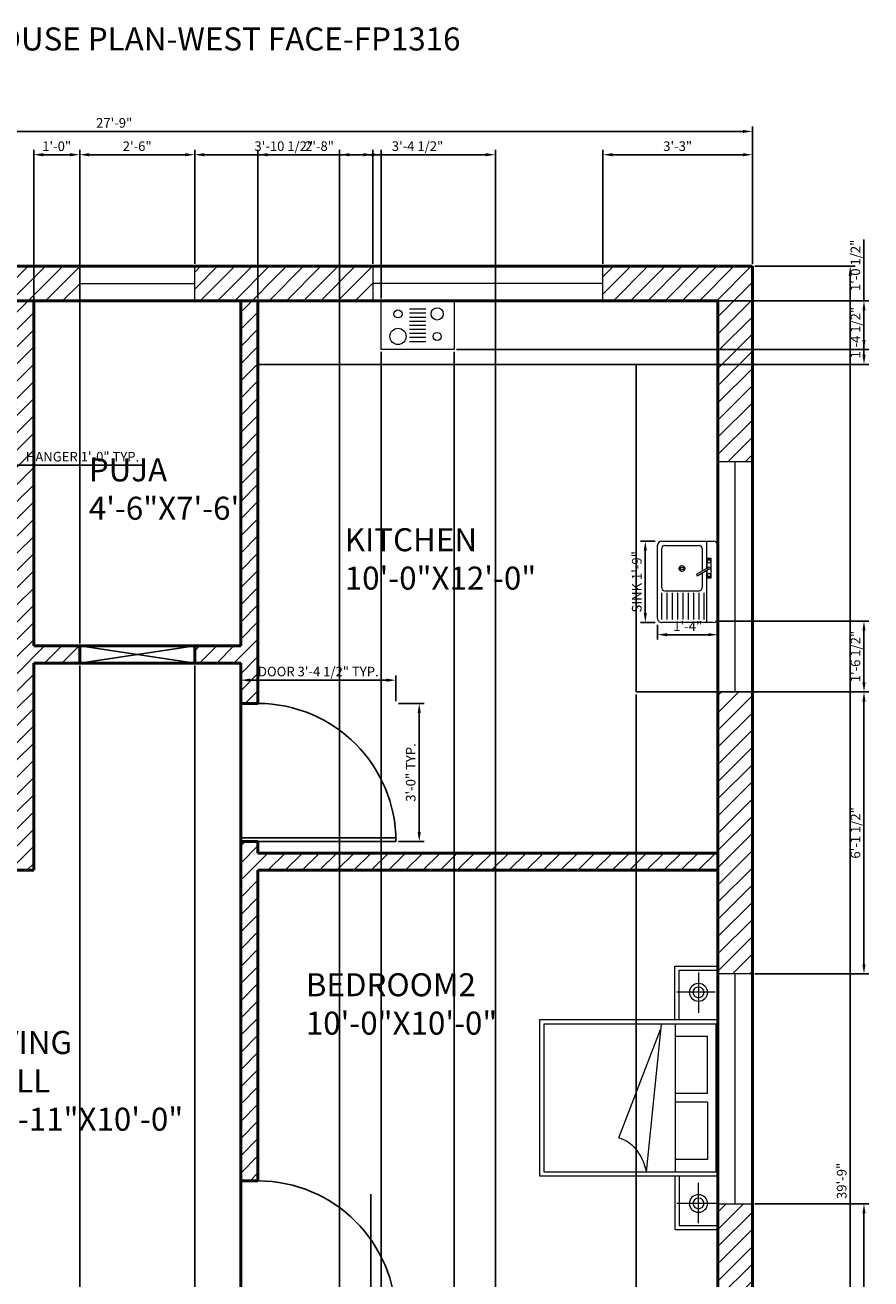
# Model space of a CAD drawing. Units: inches. Extents: x 3887 to 4286, y 884 to 1458.
# Tile 4 of 4: x 4065 to 4286, y 1131 to 1458. Entities that reach past the tile are written whole.
import ezdxf

# ---------------------------------------------------------------- set-up
doc = ezdxf.new("R2010")
doc.units = ezdxf.units.IN
for name, color, linetype, lineweight in [('A-ANNO-DIMS', 2, 'Continuous', 18), ('A-ANNO-TEXT', 7, 'Continuous', 25), ('A-AREA-IDEN', 7, 'Continuous', 25), ('A-DOOR', 3, 'Continuous', 25), ('A-EQPM', 9, 'Continuous', 18), ('A-FLOR-CASE', 8, 'Continuous', 25), ('A-FLOR-FIXT', 8, 'Continuous', 18), ('A-FURN', 8, 'Continuous', 18), ('A-GLAZ', 4, 'Continuous', 18), ('A-WALL', 7, 'Continuous', 50), ('A-WALL-PATT', 252, 'Continuous', 13)]:
    doc.layers.add(name, color=color, linetype=linetype, lineweight=lineweight)
doc.styles.get("Standard").update_dxf_attribs({"font": 'arial.ttf'})
doc.dimstyles.new('ISO-25', dxfattribs={"dimtxt": 2.5, "dimasz": 2.5, "dimexe": 1.25, "dimexo": 0.625, "dimtad": 1, "dimdec": 0, "dimlunit": 3, "dimtxsty": 'Standard', "dimcen": 2.5, "dimadec": 0, "dimazin": 0, "dimtfac": 1, "dimtdec": 0, "dimtmove": 0, "dimatfit": 3, "dimfxl": 1, "dimarcsym": 0})

# ---------------------------------------------------------------- blocks, each defined once
blk = doc.blocks.new('kitchen sink 1')
at = {"color": 0}
for p, q in [((-345, -98), (-112, -98)), ((-195, -72), (-195, -79)), ((-187, -72), (-195, -72)), ((-195, -79), (-187, -79)), ((-118, -86), (-65, -178)), ((-53, -170), (-106, -79)), ((-95, -98), (345, -98)), ((-46, -72), (-38, -72)), ((-38, -79), (-46, -79)), ((-38, -72), (-38, -79)), ((76, -452), (76, -159)), ((94, -118), (319, -118)), ((94, -163), (319, -163)), ((94, -208), (319, -208)), ((94, -253), (319, -253)), ((94, -298), (319, -298)), ((94, -343), (319, -343)), ((94, -388), (319, -388)), ((94, -433), (319, -433)), ((94, -478), (319, -478))]:
    blk.add_line(p, q, dxfattribs=at)
for points in [[(-309, 0), (309, 0)], [(-345, -476), (-345, -37)], [(-116, -90), (-202, -90), (-202, -61), (-31, -61), (-31, -90), (-100, -90)], [(345, -37), (345, -476)], [(-309, -452), (-309, -159)], [(-284, -134), (-90, -134)], [(-74, -134), (52, -134)], [(309, -513), (-309, -513)], [(52, -476), (-284, -476)]]:
    blk.add_lwpolyline(points, dxfattribs=at)
for centre, radius in [((-173, -75), 14.3), ((-116, -75), 10.7), ((-59, -75), 14.3), ((-113, -305), 24.4), ((-113, -305), 12.2)]:
    blk.add_circle(centre, radius, dxfattribs=at)
for centre, radius, start, end in [((-309, -37), 36.6, 90, 180), ((309, -37), 36.6, 0, 90), ((-284, -159), 24.4, 90, 180), ((-59, -174), 7.13, 210, 30), ((52, -159), 24.4, 0, 90), ((-309, -476), 36.6, 180, 270), ((-284, -452), 24.4, 180, 270), ((52, -452), 24.4, 270, 0), ((309, -476), 36.6, 270, 0)]:
    blk.add_arc(centre, radius, start, end, dxfattribs=at)
blk = doc.blocks.new('*D10')
at = {"layer": 'A-ANNO-DIMS', "color": 0, "lineweight": -2, "transparency": 16777216}
for p, q in [((3922.18, 1395.27), (3922.18, 1431.07)), ((3924.68, 1429.82), (4252.68, 1429.82)), ((4255.18, 1395.27), (4255.18, 1431.07))]:
    blk.add_line(p, q, dxfattribs=at)
at = {"layer": 'A-ANNO-DIMS', "color": 0, "transparency": 16777216}
for points in [[(3924.68, 1430.23), (3924.68, 1429.4), (3922.18, 1429.82)], [(4252.68, 1430.23), (4252.68, 1429.4), (4255.18, 1429.82)]]:
    blk.add_solid(points, dxfattribs=at)
at = {"layer": 'Defpoints', "color": 0, "transparency": 16777216}
for p in [(4255.18, 1429.82), (3922.18, 1394.64), (4255.18, 1394.64)]:
    blk.add_point(p, dxfattribs=at)
at = {"layer": 'A-ANNO-DIMS', "color": 0, "transparency": 16777216, "insert": (4088.68, 1431.72), "char_height": 2.5, "attachment_point": 5}
blk.add_mtext('27\'-9"', dxfattribs=at)
blk = doc.blocks.new('*D11')
at = {"layer": 'A-ANNO-DIMS', "color": 0, "lineweight": -2, "transparency": 16777216}
for p, q in [((4255.81, 1394.64), (4281.94, 1394.64)), ((4280.69, 1392.14), (4280.69, 920.14)), ((4255.81, 917.64), (4281.94, 917.64))]:
    blk.add_line(p, q, dxfattribs=at)
at = {"layer": 'A-ANNO-DIMS', "color": 0, "transparency": 16777216}
for points in [[(4280.27, 1392.14), (4281.11, 1392.14), (4280.69, 1394.64)], [(4280.27, 920.14), (4281.11, 920.14), (4280.69, 917.64)]]:
    blk.add_solid(points, dxfattribs=at)
at = {"layer": 'Defpoints', "color": 0, "transparency": 16777216}
for p in [(4255.18, 1394.64), (4255.18, 917.64), (4280.69, 917.64)]:
    blk.add_point(p, dxfattribs=at)
at = {"layer": 'A-ANNO-DIMS', "color": 0, "transparency": 16777216, "insert": (4278.79, 1156.14), "char_height": 2.5, "attachment_point": 5, "rotation": 90}
blk.add_mtext('39\'-9"', dxfattribs=at)
blk = doc.blocks.new('DOOR-SWING-36IN')
for p, q in [((35, 0), (35, 40.5)), ((36, 4.5), (36, 40.5))]:
    blk.add_line(p, q)
blk.add_arc((36, 4.5), 36, 90, 180)
blk = doc.blocks.new('WIN-GLAZ-60IN')
for p, q in [((60, 9), (0, 9)), ((0, 4.5), (60, 4.5)), ((0, 0), (60, 0))]:
    blk.add_line(p, q)
blk = doc.blocks.new('*D15')
at = {"layer": 'A-ANNO-DIMS', "color": 0, "lineweight": -2, "transparency": 16777216}
for p, q in [((4049.91, 1341.61), (4049.91, 1344.01)), ((4061.79, 1341.61), (4061.79, 1344.01)), ((4052.41, 1342.76), (4059.29, 1342.76)), ((4061.79, 1342.76), (4096.55, 1342.76))]:
    blk.add_line(p, q, dxfattribs=at)
at = {"layer": 'A-ANNO-DIMS', "color": 0, "transparency": 16777216}
for points in [[(4052.41, 1343.18), (4052.41, 1342.35), (4049.91, 1342.76)], [(4059.29, 1343.18), (4059.29, 1342.35), (4061.79, 1342.76)]]:
    blk.add_solid(points, dxfattribs=at)
at = {"layer": 'Defpoints', "color": 0, "transparency": 16777216}
for p in [(4049.91, 1340.98), (4061.79, 1342.76), (4061.79, 1340.98)]:
    blk.add_point(p, dxfattribs=at)
at = {"layer": 'A-ANNO-DIMS', "color": 0, "transparency": 16777216, "insert": (4080.42, 1344.68), "char_height": 2.5, "attachment_point": 5}
blk.add_mtext('HANGER 1\'-0" TYP.', dxfattribs=at)
blk = doc.blocks.new('*D19')
at = {"layer": 'A-ANNO-DIMS', "color": 0, "lineweight": -2, "transparency": 16777216}
for p, q in [((4121.68, 1281.27), (4121.68, 1287.97)), ((4124.18, 1286.72), (4159.68, 1286.72)), ((4162.18, 1281.27), (4162.18, 1287.97))]:
    blk.add_line(p, q, dxfattribs=at)
at = {"layer": 'A-ANNO-DIMS', "color": 0, "transparency": 16777216}
for points in [[(4124.18, 1287.14), (4124.18, 1286.3), (4121.68, 1286.72)], [(4159.68, 1287.14), (4159.68, 1286.3), (4162.18, 1286.72)]]:
    blk.add_solid(points, dxfattribs=at)
at = {"layer": 'Defpoints', "color": 0, "transparency": 16777216}
for p in [(4162.18, 1286.72), (4121.68, 1280.64), (4162.18, 1280.64)]:
    blk.add_point(p, dxfattribs=at)
at = {"layer": 'A-ANNO-DIMS', "color": 0, "transparency": 16777216, "insert": (4141.93, 1288.64), "char_height": 2.5, "attachment_point": 5}
blk.add_mtext('DOOR 3\'-4 1/2" TYP.', dxfattribs=at)
blk = doc.blocks.new('*D20')
at = {"layer": 'A-ANNO-DIMS', "color": 0, "lineweight": -2, "transparency": 16777216}
for p, q in [((4162.81, 1280.64), (4169.51, 1280.64)), ((4168.26, 1278.14), (4168.26, 1247.14)), ((4162.81, 1244.64), (4169.51, 1244.64))]:
    blk.add_line(p, q, dxfattribs=at)
at = {"layer": 'A-ANNO-DIMS', "color": 0, "transparency": 16777216}
for points in [[(4167.84, 1278.14), (4168.68, 1278.14), (4168.26, 1280.64)], [(4167.84, 1247.14), (4168.68, 1247.14), (4168.26, 1244.64)]]:
    blk.add_solid(points, dxfattribs=at)
at = {"layer": 'Defpoints', "color": 0, "transparency": 16777216}
for p in [(4162.18, 1280.64), (4162.18, 1244.64), (4168.26, 1244.64)]:
    blk.add_point(p, dxfattribs=at)
at = {"layer": 'A-ANNO-DIMS', "color": 0, "transparency": 16777216, "insert": (4166.36, 1262.64), "char_height": 2.5, "attachment_point": 5, "rotation": 90}
blk.add_mtext('3\'-0" TYP.', dxfattribs=at)
blk = doc.blocks.new('*D23')
at = {"layer": 'A-ANNO-DIMS', "color": 0, "lineweight": -2, "transparency": 16777216}
for p, q in [((4229.79, 1322.97), (4225.99, 1322.97)), ((4227.24, 1320.47), (4227.24, 1304.26)), ((4229.79, 1301.76), (4225.99, 1301.76))]:
    blk.add_line(p, q, dxfattribs=at)
at = {"layer": 'A-ANNO-DIMS', "color": 0, "transparency": 16777216}
for points in [[(4226.82, 1320.47), (4227.65, 1320.47), (4227.24, 1322.97)], [(4226.82, 1304.26), (4227.65, 1304.26), (4227.24, 1301.76)]]:
    blk.add_solid(points, dxfattribs=at)
at = {"layer": 'Defpoints', "color": 0, "transparency": 16777216}
for p in [(4230.42, 1322.97), (4227.24, 1301.76), (4230.42, 1301.76)]:
    blk.add_point(p, dxfattribs=at)
at = {"layer": 'A-ANNO-DIMS', "color": 0, "transparency": 16777216, "insert": (4225.32, 1312.37), "char_height": 2.5, "attachment_point": 5, "rotation": 90}
blk.add_mtext('SINK 1\'-9"', dxfattribs=at)
blk = doc.blocks.new('*D24')
at = {"layer": 'A-ANNO-DIMS', "color": 0, "lineweight": -2, "transparency": 16777216}
for p, q in [((4230.42, 1301.14), (4230.42, 1297.33)), ((4232.92, 1298.58), (4243.67, 1298.58)), ((4246.17, 1301.14), (4246.17, 1297.33))]:
    blk.add_line(p, q, dxfattribs=at)
at = {"layer": 'A-ANNO-DIMS', "color": 0, "transparency": 16777216}
for points in [[(4232.92, 1299), (4232.92, 1298.16), (4230.42, 1298.58)], [(4243.67, 1299), (4243.67, 1298.16), (4246.17, 1298.58)]]:
    blk.add_solid(points, dxfattribs=at)
at = {"layer": 'Defpoints', "color": 0, "transparency": 16777216}
for p in [(4230.42, 1301.76), (4246.17, 1301.76), (4246.17, 1298.58)]:
    blk.add_point(p, dxfattribs=at)
at = {"layer": 'A-ANNO-DIMS', "color": 0, "transparency": 16777216, "insert": (4238.3, 1300.46), "char_height": 2.5, "attachment_point": 5}
blk.add_mtext('1\'-4"', dxfattribs=at)
blk = doc.blocks.new('*D34')
at = {"layer": 'A-ANNO-DIMS', "color": 0, "lineweight": -2, "transparency": 16777216}
for p, q in [((4255.81, 1150.14), (4285.53, 1150.14)), ((4284.28, 1076.14), (4284.28, 1147.64)), ((4255.81, 1073.64), (4285.53, 1073.64))]:
    blk.add_line(p, q, dxfattribs=at)
at = {"layer": 'A-ANNO-DIMS', "color": 0, "transparency": 16777216}
for points in [[(4283.87, 1147.64), (4284.7, 1147.64), (4284.28, 1150.14)], [(4283.87, 1076.14), (4284.7, 1076.14), (4284.28, 1073.64)]]:
    blk.add_solid(points, dxfattribs=at)
at = {"layer": 'Defpoints', "color": 0, "transparency": 16777216}
for p in [(4255.18, 1150.14), (4284.28, 1150.14), (4255.18, 1073.64)]:
    blk.add_point(p, dxfattribs=at)
at = {"layer": 'A-ANNO-DIMS', "color": 0, "transparency": 16777216, "insert": (4282.37, 1111.89), "char_height": 2.5, "attachment_point": 5, "rotation": 90}
blk.add_mtext('6\'-4 1/2"', dxfattribs=at)
blk = doc.blocks.new('*D35')
at = {"layer": 'A-ANNO-DIMS', "color": 0, "lineweight": -2, "transparency": 16777216}
for p, q in [((4255.81, 1283.64), (4285.53, 1283.64)), ((4284.28, 1212.64), (4284.28, 1281.14)), ((4255.81, 1210.14), (4285.53, 1210.14))]:
    blk.add_line(p, q, dxfattribs=at)
at = {"layer": 'A-ANNO-DIMS', "color": 0, "transparency": 16777216}
for points in [[(4283.87, 1281.14), (4284.7, 1281.14), (4284.28, 1283.64)], [(4283.87, 1212.64), (4284.7, 1212.64), (4284.28, 1210.14)]]:
    blk.add_solid(points, dxfattribs=at)
at = {"layer": 'Defpoints', "color": 0, "transparency": 16777216}
for p in [(4255.18, 1283.64), (4284.28, 1283.64), (4255.18, 1210.14)]:
    blk.add_point(p, dxfattribs=at)
at = {"layer": 'A-ANNO-DIMS', "color": 0, "transparency": 16777216, "insert": (4282.37, 1246.89), "char_height": 2.5, "attachment_point": 5, "rotation": 90}
blk.add_mtext('6\'-1 1/2"', dxfattribs=at)
blk = doc.blocks.new('*D36')
at = {"layer": 'A-ANNO-DIMS', "color": 0, "lineweight": -2, "transparency": 16777216}
for p, q in [((4216.18, 1395.27), (4216.18, 1424.99)), ((4218.68, 1423.74), (4252.68, 1423.74)), ((4255.18, 1395.27), (4255.18, 1424.99))]:
    blk.add_line(p, q, dxfattribs=at)
at = {"layer": 'A-ANNO-DIMS', "color": 0, "transparency": 16777216}
for points in [[(4218.68, 1424.16), (4218.68, 1423.33), (4216.18, 1423.74)], [(4252.68, 1424.16), (4252.68, 1423.33), (4255.18, 1423.74)]]:
    blk.add_solid(points, dxfattribs=at)
at = {"layer": 'Defpoints', "color": 0, "transparency": 16777216}
for p in [(4255.18, 1423.74), (4216.18, 1394.64), (4255.18, 1394.64)]:
    blk.add_point(p, dxfattribs=at)
at = {"layer": 'A-ANNO-DIMS', "color": 0, "transparency": 16777216, "insert": (4235.68, 1425.65), "char_height": 2.5, "attachment_point": 5}
blk.add_mtext('3\'-3"', dxfattribs=at)
blk = doc.blocks.new('*D37')
at = {"layer": 'A-ANNO-DIMS', "color": 0, "lineweight": -2, "transparency": 16777216}
for p, q in [((4109.68, 1395.27), (4109.68, 1424.99)), ((4112.18, 1423.74), (4153.68, 1423.74)), ((4156.18, 1395.27), (4156.18, 1424.99))]:
    blk.add_line(p, q, dxfattribs=at)
at = {"layer": 'A-ANNO-DIMS', "color": 0, "transparency": 16777216}
for points in [[(4112.18, 1424.16), (4112.18, 1423.33), (4109.68, 1423.74)], [(4153.68, 1424.16), (4153.68, 1423.33), (4156.18, 1423.74)]]:
    blk.add_solid(points, dxfattribs=at)
at = {"layer": 'Defpoints', "color": 0, "transparency": 16777216}
for p in [(4156.18, 1423.74), (4109.68, 1394.64), (4156.18, 1394.64)]:
    blk.add_point(p, dxfattribs=at)
at = {"layer": 'A-ANNO-DIMS', "color": 0, "transparency": 16777216, "insert": (4132.93, 1425.66), "char_height": 2.5, "attachment_point": 5}
blk.add_mtext('3\'-10 1/2"', dxfattribs=at)
blk = doc.blocks.new('*D38')
at = {"layer": 'A-ANNO-DIMS', "color": 0, "lineweight": -2, "transparency": 16777216}
for p, q in [((4079.68, 1395.27), (4079.68, 1424.99)), ((4082.18, 1423.74), (4107.18, 1423.74)), ((4109.68, 1395.27), (4109.68, 1424.99))]:
    blk.add_line(p, q, dxfattribs=at)
at = {"layer": 'A-ANNO-DIMS', "color": 0, "transparency": 16777216}
for points in [[(4082.18, 1424.16), (4082.18, 1423.33), (4079.68, 1423.74)], [(4107.18, 1424.16), (4107.18, 1423.33), (4109.68, 1423.74)]]:
    blk.add_solid(points, dxfattribs=at)
at = {"layer": 'Defpoints', "color": 0, "transparency": 16777216}
for p in [(4109.68, 1423.74), (4079.68, 1394.64), (4109.68, 1394.64)]:
    blk.add_point(p, dxfattribs=at)
at = {"layer": 'A-ANNO-DIMS', "color": 0, "transparency": 16777216, "insert": (4094.68, 1425.65), "char_height": 2.5, "attachment_point": 5}
blk.add_mtext('2\'-6"', dxfattribs=at)
blk = doc.blocks.new('*D48')
at = {"layer": 'A-ANNO-DIMS', "color": 0, "lineweight": -2, "transparency": 16777216}
for p, q in [((4147.49, 1047.25), (4147.49, 1424.99)), ((4149.99, 1423.74), (4185.63, 1423.74)), ((4188.13, 1047.25), (4188.13, 1424.99))]:
    blk.add_line(p, q, dxfattribs=at)
at = {"layer": 'A-ANNO-DIMS', "color": 0, "transparency": 16777216}
for points in [[(4149.99, 1424.16), (4149.99, 1423.33), (4147.49, 1423.74)], [(4185.63, 1424.16), (4185.63, 1423.33), (4188.13, 1423.74)]]:
    blk.add_solid(points, dxfattribs=at)
at = {"layer": 'Defpoints', "color": 0, "transparency": 16777216}
for p in [(4188.13, 1423.74), (4147.49, 1046.63), (4188.13, 1046.63)]:
    blk.add_point(p, dxfattribs=at)
at = {"layer": 'A-ANNO-DIMS', "color": 0, "transparency": 16777216, "insert": (4167.81, 1425.66), "char_height": 2.5, "attachment_point": 5}
blk.add_mtext('3\'-4 1/2"', dxfattribs=at)
blk = doc.blocks.new('*D50')
at = {"layer": 'A-ANNO-DIMS', "color": 0, "lineweight": -2, "transparency": 16777216}
for p, q in [((4224.82, 1283.02), (4224.82, 887.29)), ((4246.18, 1283.02), (4246.18, 887.29)), ((4227.32, 888.54), (4243.68, 888.54))]:
    blk.add_line(p, q, dxfattribs=at)
at = {"layer": 'A-ANNO-DIMS', "color": 0, "transparency": 16777216}
for points in [[(4227.32, 888.96), (4227.32, 888.13), (4224.82, 888.54)], [(4243.68, 888.96), (4243.68, 888.13), (4246.18, 888.54)]]:
    blk.add_solid(points, dxfattribs=at)
at = {"layer": 'Defpoints', "color": 0, "transparency": 16777216}
for p in [(4224.82, 1283.64), (4246.18, 1283.64), (4246.18, 888.54)]:
    blk.add_point(p, dxfattribs=at)
at = {"layer": 'A-ANNO-DIMS', "color": 0, "transparency": 16777216, "insert": (4235.5, 890.46), "char_height": 2.5, "attachment_point": 5}
blk.add_mtext('1\'-9 1/2"', dxfattribs=at)
blk = doc.blocks.new('*D51')
at = {"layer": 'A-ANNO-DIMS', "color": 0, "lineweight": -2, "transparency": 16777216}
for p, q in [((4126.81, 1385.64), (4285.53, 1385.64)), ((4284.28, 1371.58), (4284.28, 1383.14)), ((4126.81, 1369.08), (4285.53, 1369.08))]:
    blk.add_line(p, q, dxfattribs=at)
at = {"layer": 'A-ANNO-DIMS', "color": 0, "transparency": 16777216}
for points in [[(4283.87, 1383.14), (4284.7, 1383.14), (4284.28, 1385.64)], [(4283.87, 1371.58), (4284.7, 1371.58), (4284.28, 1369.08)]]:
    blk.add_solid(points, dxfattribs=at)
at = {"layer": 'Defpoints', "color": 0, "transparency": 16777216}
for p in [(4126.18, 1385.64), (4284.28, 1385.64), (4126.18, 1369.08)]:
    blk.add_point(p, dxfattribs=at)
at = {"layer": 'A-ANNO-DIMS', "color": 0, "transparency": 16777216, "insert": (4282.37, 1377.36), "char_height": 2.5, "attachment_point": 5, "rotation": 90}
blk.add_mtext('1\'-4 1/2"', dxfattribs=at)
blk = doc.blocks.new('*D54')
at = {"layer": 'A-ANNO-DIMS', "color": 0, "lineweight": -2, "transparency": 16777216}
for p, q in [((4158.31, 1372.33), (4158.31, 887.29)), ((4177.34, 1372.33), (4177.34, 887.29)), ((4160.81, 888.54), (4174.84, 888.54))]:
    blk.add_line(p, q, dxfattribs=at)
at = {"layer": 'A-ANNO-DIMS', "color": 0, "transparency": 16777216}
for points in [[(4160.81, 888.96), (4160.81, 888.13), (4158.31, 888.54)], [(4174.84, 888.96), (4174.84, 888.13), (4177.34, 888.54)]]:
    blk.add_solid(points, dxfattribs=at)
at = {"layer": 'Defpoints', "color": 0, "transparency": 16777216}
for p in [(4158.31, 1372.95), (4177.34, 1372.95), (4177.34, 888.54)]:
    blk.add_point(p, dxfattribs=at)
at = {"layer": 'A-ANNO-DIMS', "color": 0, "transparency": 16777216, "insert": (4167.82, 890.42), "char_height": 2.5, "attachment_point": 5}
blk.add_mtext('1\'-7"', dxfattribs=at)
blk = doc.blocks.new('*D55')
at = {"layer": 'A-ANNO-DIMS', "color": 0, "lineweight": -2, "transparency": 16777216}
for p, q in [((4284.28, 1385.64), (4284.28, 1401.63)), ((4177.97, 1385.64), (4285.53, 1385.64)), ((4284.28, 1375.45), (4284.28, 1383.14)), ((4177.97, 1372.95), (4285.53, 1372.95))]:
    blk.add_line(p, q, dxfattribs=at)
at = {"layer": 'A-ANNO-DIMS', "color": 0, "transparency": 16777216}
for points in [[(4283.87, 1383.14), (4284.7, 1383.14), (4284.28, 1385.64)], [(4283.87, 1375.45), (4284.7, 1375.45), (4284.28, 1372.95)]]:
    blk.add_solid(points, dxfattribs=at)
at = {"layer": 'Defpoints', "color": 0, "transparency": 16777216}
for p in [(4177.34, 1385.64), (4284.28, 1385.64), (4177.34, 1372.95)]:
    blk.add_point(p, dxfattribs=at)
at = {"layer": 'A-ANNO-DIMS', "color": 0, "transparency": 16777216, "insert": (4282.37, 1394.89), "char_height": 2.5, "attachment_point": 5, "rotation": 90}
blk.add_mtext('1\'-0 1/2"', dxfattribs=at)
blk = doc.blocks.new('*D56')
at = {"layer": 'A-ANNO-DIMS', "color": 0, "lineweight": -2, "transparency": 16777216}
for p, q in [((4126.18, 1386.27), (4126.18, 1424.99)), ((4128.68, 1423.74), (4155.81, 1423.74)), ((4158.31, 1386.27), (4158.31, 1424.99))]:
    blk.add_line(p, q, dxfattribs=at)
at = {"layer": 'A-ANNO-DIMS', "color": 0, "transparency": 16777216}
for points in [[(4128.68, 1424.16), (4128.68, 1423.33), (4126.18, 1423.74)], [(4155.81, 1424.16), (4155.81, 1423.33), (4158.31, 1423.74)]]:
    blk.add_solid(points, dxfattribs=at)
at = {"layer": 'Defpoints', "color": 0, "transparency": 16777216}
for p in [(4158.31, 1423.74), (4126.18, 1385.64), (4158.31, 1385.64)]:
    blk.add_point(p, dxfattribs=at)
at = {"layer": 'A-ANNO-DIMS', "color": 0, "transparency": 16777216, "insert": (4142.24, 1425.65), "char_height": 2.5, "attachment_point": 5}
blk.add_mtext('2\'-8"', dxfattribs=at)
blk = doc.blocks.new('*D57')
at = {"layer": 'A-ANNO-DIMS', "color": 0, "lineweight": -2, "transparency": 16777216}
for p, q in [((4246.47, 1302.09), (4285.53, 1302.09)), ((4284.28, 1286.14), (4284.28, 1299.59)), ((4246.81, 1283.64), (4285.53, 1283.64))]:
    blk.add_line(p, q, dxfattribs=at)
at = {"layer": 'A-ANNO-DIMS', "color": 0, "transparency": 16777216}
for points in [[(4283.87, 1299.59), (4284.7, 1299.59), (4284.28, 1302.09)], [(4283.87, 1286.14), (4284.7, 1286.14), (4284.28, 1283.64)]]:
    blk.add_solid(points, dxfattribs=at)
at = {"layer": 'Defpoints', "color": 0, "transparency": 16777216}
for p in [(4245.84, 1302.09), (4284.28, 1302.09), (4246.18, 1283.64)]:
    blk.add_point(p, dxfattribs=at)
at = {"layer": 'A-ANNO-DIMS', "color": 0, "transparency": 16777216, "insert": (4282.37, 1292.87), "char_height": 2.5, "attachment_point": 5, "rotation": 90}
blk.add_mtext('1\'-6 1/2"', dxfattribs=at)
blk = doc.blocks.new('*D58')
at = {"layer": 'A-ANNO-DIMS', "color": 0, "lineweight": -2, "transparency": 16777216}
for p, q in [((4067.68, 1296.27), (4067.68, 1424.99)), ((4070.18, 1423.74), (4077.18, 1423.74)), ((4079.68, 1296.27), (4079.68, 1424.99))]:
    blk.add_line(p, q, dxfattribs=at)
at = {"layer": 'A-ANNO-DIMS', "color": 0, "transparency": 16777216}
for points in [[(4070.18, 1424.16), (4070.18, 1423.33), (4067.68, 1423.74)], [(4077.18, 1424.16), (4077.18, 1423.33), (4079.68, 1423.74)]]:
    blk.add_solid(points, dxfattribs=at)
at = {"layer": 'Defpoints', "color": 0, "transparency": 16777216}
for p in [(4079.68, 1423.74), (4067.68, 1295.64), (4079.68, 1295.64)]:
    blk.add_point(p, dxfattribs=at)
at = {"layer": 'A-ANNO-DIMS', "color": 0, "transparency": 16777216, "insert": (4073.68, 1425.65), "char_height": 2.5, "attachment_point": 5}
blk.add_mtext('1\'-0"', dxfattribs=at)
blk = doc.blocks.new('*D59')
at = {"layer": 'A-ANNO-DIMS', "color": 0, "lineweight": -2, "transparency": 16777216}
for p, q in [((4079.68, 1290.52), (4079.68, 887.29)), ((4109.68, 1290.52), (4109.68, 887.29)), ((4082.18, 888.54), (4107.18, 888.54))]:
    blk.add_line(p, q, dxfattribs=at)
at = {"layer": 'A-ANNO-DIMS', "color": 0, "transparency": 16777216}
for points in [[(4082.18, 888.96), (4082.18, 888.13), (4079.68, 888.54)], [(4107.18, 888.96), (4107.18, 888.13), (4109.68, 888.54)]]:
    blk.add_solid(points, dxfattribs=at)
at = {"layer": 'Defpoints', "color": 0, "transparency": 16777216}
for p in [(4079.68, 1291.14), (4109.68, 1291.14), (4109.68, 888.54)]:
    blk.add_point(p, dxfattribs=at)
at = {"layer": 'A-ANNO-DIMS', "color": 0, "transparency": 16777216, "insert": (4094.68, 890.45), "char_height": 2.5, "attachment_point": 5}
blk.add_mtext('2\'-6"', dxfattribs=at)
blk = doc.blocks.new('*D60')
at = {"layer": 'A-ANNO-DIMS', "color": 0, "lineweight": -2, "transparency": 16777216}
for p, q in [((4155.6, 1152.64), (4155.6, 1091.64)), ((4155.6, 1049.9), (4155.6, 1089.14))]:
    blk.add_line(p, q, dxfattribs=at)
at = {"layer": 'A-ANNO-DIMS', "color": 0, "transparency": 16777216}
blk.add_solid([(4155.18, 1089.14), (4156.01, 1089.14), (4155.6, 1091.64)], dxfattribs=at)
at = {"layer": 'Defpoints', "color": 0, "transparency": 16777216}
for p in [(4155.6, 1152.64), (4155.6, 1091.64)]:
    blk.add_point(p, dxfattribs=at)
at = {"layer": 'A-ANNO-DIMS', "color": 0, "transparency": 16777216, "insert": (4153.7, 1055.04), "char_height": 2.5, "attachment_point": 5, "rotation": 90}
blk.add_mtext('R5\'-1"', dxfattribs=at)

msp = doc.modelspace()

# ---------------------------------------------------------------- hatches: boundary and pattern name
at = {"layer": 'A-WALL-PATT'}
h = msp.add_hatch(dxfattribs=at)
h.set_pattern_fill('ANSI31', color=256)
h.paths.add_polyline_path([(4079.68, 1394.64), (3922.18, 1394.64), (3922.18, 1343.64), (3931.18, 1343.64), (3931.18, 1385.64), (4079.68, 1385.64)])
h.paths.add_polyline_path([(4156.18, 1394.64), (4109.68, 1394.64), (4109.68, 1385.64), (4156.18, 1385.64)])
h.paths.add_polyline_path([(4255.18, 1394.64), (4216.18, 1394.64), (4216.18, 1385.64), (4246.18, 1385.64), (4246.18, 1343.64), (4255.18, 1343.64)])
h.paths.add_polyline_path([(3931.18, 1283.64), (3922.18, 1283.64), (3922.18, 1207.14), (3931.18, 1207.14)])
h.paths.add_polyline_path([(4024.18, 1241.64), (3931.18, 1241.64), (3931.18, 1237.14), (4024.18, 1237.14)])
h.paths.add_polyline_path([(4067.68, 1291.14), (4079.68, 1291.14), (4079.68, 1295.64), (4067.68, 1295.64), (4067.68, 1385.64), (4063.18, 1385.64), (4063.18, 1241.64), (4060.18, 1241.64), (4060.18, 1237.14), (4067.68, 1237.14)])
h.paths.add_polyline_path([(4126.18, 1385.64), (4121.68, 1385.64), (4121.68, 1295.64), (4109.68, 1295.64), (4109.68, 1291.14), (4121.68, 1291.14), (4121.68, 1280.64), (4126.18, 1280.64)])
h.paths.add_polyline_path([(4246.18, 1241.64), (4126.18, 1241.64), (4126.18, 1244.64), (4121.68, 1244.64), (4121.68, 1156.14), (4126.18, 1156.14), (4126.18, 1237.14), (4246.18, 1237.14)])
h.paths.add_polyline_path([(4255.18, 1283.64), (4246.18, 1283.64), (4246.18, 1210.14), (4255.18, 1210.14)])
h.paths.add_polyline_path([(4255.18, 1150.14), (4246.18, 1150.14), (4246.18, 1073.64), (4255.18, 1073.64)])
h.paths.add_polyline_path([(4246.18, 1117.14), (4126.18, 1117.14), (4126.18, 1120.14), (4121.68, 1120.14), (4121.68, 1117.14), (4119.68, 1117.14), (4119.68, 1112.64), (4246.18, 1112.64)])
h.paths.add_polyline_path([(4079.18, 1112.64), (4083.68, 1112.64), (4083.68, 1117.14), (4074.68, 1117.14), (4074.68, 974.64), (4079.18, 974.64)])
h.paths.add_polyline_path([(4019.68, 1117.14), (3970.18, 1117.14), (3970.18, 1112.64), (4015.18, 1112.64), (4015.18, 974.64), (4019.68, 974.64), (4019.68, 1058.64), (4021.68, 1058.64), (4021.68, 1063.14), (4019.68, 1063.14)])
h.paths.add_polyline_path([(3931.18, 1147.14), (3922.18, 1147.14), (3922.18, 917.64), (3933.18, 917.64), (3933.18, 926.64), (3931.18, 926.64)])
h.paths.add_polyline_path([(4024.18, 965.64), (4036.18, 965.64), (4036.18, 974.64), (4015.18, 974.64), (4015.18, 926.64), (4003.18, 926.64), (4003.18, 917.64), (4024.18, 917.64)])
h.paths.add_polyline_path([(4132.68, 974.64), (4062.68, 974.64), (4062.68, 965.64), (4132.68, 965.64)])
h.paths.add_polyline_path([(4255.18, 1013.64), (4246.18, 1013.64), (4246.18, 974.64), (4192.68, 974.64), (4192.68, 965.64), (4255.18, 965.64)])

# ---------------------------------------------------------------- linework, layer by layer
at = {"layer": 'A-DOOR'}
for p, q in [((4079.68, 1295.64), (4109.68, 1291.14)), ((4079.68, 1291.14), (4109.68, 1295.64))]:
    msp.add_line(p, q, dxfattribs=at)
at = {"layer": 'A-EQPM'}
for p, q in [((4165.71, 1383.53), (4169.94, 1383.53)), ((4165.71, 1382.47), (4169.94, 1382.47)), ((4165.71, 1381.41), (4169.94, 1381.41)), ((4165.71, 1380.36), (4169.94, 1380.36)), ((4165.71, 1379.3), (4169.94, 1379.3)), ((4165.71, 1378.24), (4169.94, 1378.24)), ((4165.71, 1377.18), (4169.94, 1377.18)), ((4165.71, 1376.13), (4169.94, 1376.13)), ((4165.71, 1375.07), (4169.94, 1375.07))]:
    msp.add_line(p, q, dxfattribs=at)
msp.add_lwpolyline([(4158.31, 1372.95), (4158.31, 1385.64), (4177.34, 1385.64), (4177.34, 1372.95)], close=True, dxfattribs=at)
for centre, radius in [((4162.72, 1382.23), 1.06), ((4172.93, 1382.23), 1.59), ((4162.72, 1376.36), 2.12), ((4172.93, 1376.36), 1.06)]:
    msp.add_circle(centre, radius, dxfattribs=at)
at = {"layer": 'A-FLOR-CASE'}
for p, q in [((4126.18, 1369.08), (4224.82, 1369.08)), ((4224.82, 1369.08), (4224.82, 1283.64)), ((4224.82, 1283.64), (4246.18, 1283.64))]:
    msp.add_line(p, q, dxfattribs=at)
at = {"layer": 'A-FURN'}
for p, q in [((4234.94, 1212.13), (4246.18, 1212.13)), ((4234.94, 1198.2), (4234.94, 1212.13)), ((4236.06, 1211.06), (4246.18, 1211.06)), ((4236.06, 1198.2), (4236.06, 1211.06)), ((4241.11, 1210.46), (4241.11, 1199.97)), ((4246.18, 1212.13), (4246.18, 1143.43)), ((4245.48, 1205.32), (4235.49, 1205.32)), ((4199.63, 1198.13), (4199.63, 1157.43)), ((4246.18, 1198.13), (4199.63, 1198.13)), ((4200.76, 1197.05), (4200.76, 1158.53)), ((4245.73, 1197.05), (4200.76, 1197.05)), ((4231.38, 1197.04), (4227.48, 1158.51)), ((4235.09, 1158.54), (4235.09, 1197.06)), ((4245.73, 1158.53), (4245.73, 1197.05)), ((4220.31, 1167.38), (4231.24, 1195.58)), ((4243.49, 1193.84), (4235.09, 1193.84)), ((4243.49, 1178.95), (4243.49, 1193.84)), ((4243.49, 1178.95), (4235.01, 1178.95)), ((4243.49, 1176.63), (4235.01, 1176.63)), ((4243.49, 1176.63), (4243.49, 1161.74)), ((4243.49, 1161.74), (4235.09, 1161.74)), ((4200.76, 1158.53), (4245.73, 1158.53)), ((4199.63, 1157.43), (4246.18, 1157.43)), ((4234.94, 1157.35), (4234.94, 1143.43)), ((4236.06, 1157.35), (4236.06, 1144.5)), ((4241.11, 1145.12), (4241.11, 1155.61)), ((4245.73, 1150.26), (4235.49, 1150.26)), ((4236.06, 1144.5), (4246.18, 1144.5)), ((4234.94, 1143.43), (4246.18, 1143.43))]:
    msp.add_line(p, q, dxfattribs=at)
at = {"layer": 'A-FURN', "extrusion": (0, 0, -1)}
for centre in [(4241.11, 1205.32), (4241.11, 1150.26)]:
    msp.add_ellipse(centre, major_axis=(-2.4, 0), ratio=0.952381, dxfattribs=at)
for centre, major_axis, ratio, start_param, end_param in [((4241.11, 1205.32), (-1.44, 0), 0.952381, 3.141593, 9.424778), ((4218.82, 1154.59), (0, -12.97), 0.700439, 3.305513, 4.405354), ((4241.11, 1150.26), (-1.44, 0), 0.952381, 3.141593, 9.424778)]:
    msp.add_ellipse(centre, major_axis=major_axis, ratio=ratio, start_param=start_param, end_param=end_param, dxfattribs=at)
at = {"layer": 'A-GLAZ'}
for p, q in [((4079.68, 1385.64), (4079.68, 1394.64)), ((4109.68, 1385.64), (4109.68, 1394.64)), ((4156.18, 1394.64), (4156.18, 1385.64)), ((4216.18, 1385.64), (4216.18, 1394.64)), ((4079.68, 1390.14), (4109.68, 1390.14)), ((4255.18, 1343.64), (4246.18, 1343.64)), ((4246.18, 1283.64), (4255.18, 1283.64)), ((4255.18, 1210.14), (4246.18, 1210.14)), ((4246.18, 1150.14), (4255.18, 1150.14))]:
    msp.add_line(p, q, dxfattribs=at)
at = {"layer": 'A-WALL'}
for p, q in [((3922.18, 1394.64), (4255.18, 1394.64)), ((4255.18, 1394.64), (4255.18, 917.64)), ((3931.18, 1385.64), (4246.18, 1385.64)), ((4067.68, 1385.64), (4067.68, 1295.64)), ((4121.68, 1385.64), (4121.68, 1295.64)), ((4126.18, 1385.64), (4126.18, 1280.64)), ((4246.18, 1385.64), (4246.18, 974.64)), ((4067.68, 1295.64), (4121.68, 1295.64)), ((4079.68, 1295.64), (4079.68, 1291.14)), ((4109.68, 1295.64), (4109.68, 1291.14)), ((4067.68, 1291.14), (4121.68, 1291.14)), ((4067.68, 1291.14), (4067.68, 1237.14)), ((4121.68, 1291.14), (4121.68, 1117.14)), ((4121.68, 1280.64), (4126.18, 1280.64)), ((4126.18, 1244.64), (4121.68, 1244.64)), ((4126.18, 1244.64), (4126.18, 1241.64)), ((4126.18, 1241.64), (4246.18, 1241.64)), ((3931.18, 1237.14), (4067.68, 1237.14)), ((4126.18, 1237.14), (4246.18, 1237.14)), ((4126.18, 1237.14), (4126.18, 1156.14)), ((4121.68, 1156.14), (4126.18, 1156.14))]:
    msp.add_line(p, q, dxfattribs=at)

# ---------------------------------------------------------------- block references
at = {"layer": 'A-DOOR'}
for p, rotation in [((4121.68, 1280.64), 270.0000000000005), ((4121.68, 1156.14), 269.9999999999992)]:
    msp.add_blockref('DOOR-SWING-36IN', p, dxfattribs=dict(at, rotation=rotation))
at = {"layer": 'A-FLOR-FIXT', "xscale": 0.0307113977915697, "yscale": 0.0307113977915697, "zscale": 0.0307113977915697, "rotation": 270}
msp.add_blockref('kitchen sink 1', (4246.17, 1312.37), dxfattribs=at)
at = {"layer": 'A-GLAZ'}
for p, rotation in [((4216.18, 1394.64), 180), ((4255.18, 1283.64), 89.9999999999985), ((4255.18, 1150.14), 89.9999999999985)]:
    msp.add_blockref('WIN-GLAZ-60IN', p, dxfattribs=dict(at, rotation=rotation))

# ---------------------------------------------------------------- texts
at = {"layer": 'A-ANNO-TEXT', "insert": (3987.44, 1456.93), "char_height": 6, "attachment_point": 1}
msp.add_mtext_dynamic_manual_height_columns('28X40\\{1120 sq ft\\}HOUSE PLAN-WEST FACE-FP1316', width=229.9608, gutter_width=12.5, heights=[8.06], dxfattribs=at)
at = {"layer": 'A-AREA-IDEN', "char_height": 6, "attachment_point": 1}
for s, width, heights, insert in [('PUJA\\P4\'-6"X7\'-6"', 5.6608, [0], (4082.06, 1344.55)), ('KITCHEN\\P10\'-0"X12\'-0"', 17.6464, [0], (4148.83, 1326.34)), ('BEDROOM2\\P10\'-0"X10\'-0"', 52.3045, [18.45], (4138.67, 1210.29)), ('LIVING HALL\\P15\'-11"X10\'-0"', 9.7433, [0], (4052.2, 1195.24))]:
    msp.add_mtext_dynamic_manual_height_columns(s, width=width, gutter_width=12.5, heights=heights, dxfattribs=dict(at, insert=insert))

# ---------------------------------------------------------------- dimensions: what is measured, and where the dimension line sits
at = {"layer": 'A-ANNO-DIMS'}
for base, p1, p2, override, picture, middle in [((4255.18, 1429.82), (3922.18, 1394.64), (4255.18, 1394.64), {"dimclrd": 0, "dimclre": 0, "dimclrt": 0}, '*D10', (4088.68, 1431.72)), ((4156.18, 1423.74), (4109.68, 1394.64), (4156.18, 1394.64), {"dimdec": 1, "dimlfac": 1, "dimrnd": 0, "dimzin": 1, "dimdsep": 46, "dimlunit": 4, "dimfrac": 2}, '*D37', (4132.93, 1425.66)), ((4188.13, 1423.74), (4147.49, 1046.63), (4188.13, 1046.63), {"dimdec": 1, "dimlfac": 1, "dimrnd": 0, "dimzin": 1, "dimdsep": 46, "dimlunit": 4, "dimfrac": 2}, '*D48', (4167.81, 1425.66)), ((4079.68, 1423.74), (4067.68, 1295.64), (4079.68, 1295.64), {"dimdec": 1, "dimlfac": 1, "dimrnd": 0, "dimzin": 1, "dimdsep": 46, "dimlunit": 4, "dimfrac": 2}, '*D58', (4073.68, 1425.65)), ((4109.68, 1423.74), (4079.68, 1394.64), (4109.68, 1394.64), {"dimdec": 1, "dimlfac": 1, "dimrnd": 0, "dimzin": 1, "dimdsep": 46, "dimlunit": 4, "dimfrac": 2}, '*D38', (4094.68, 1425.65)), ((4158.31, 1423.74), (4126.18, 1385.64), (4158.31, 1385.64), {"dimdec": 1, "dimlfac": 1, "dimrnd": 0, "dimzin": 1, "dimdsep": 46, "dimlunit": 4, "dimfrac": 2}, '*D56', (4142.24, 1425.65)), ((4255.18, 1423.74), (4216.18, 1394.64), (4255.18, 1394.64), {"dimdec": 1, "dimlfac": 1, "dimrnd": 0, "dimzin": 1, "dimdsep": 46, "dimlunit": 4, "dimfrac": 2}, '*D36', (4235.68, 1425.65)), ((4177.34, 888.54), (4158.31, 1372.95), (4177.34, 1372.95), {"dimdec": 1, "dimlfac": 1, "dimrnd": 0, "dimzin": 1, "dimdsep": 46, "dimlunit": 4, "dimfrac": 2}, '*D54', (4167.82, 890.42)), ((4246.1736, 1298.5812), (4230.4186, 1301.7625), (4246.1736, 1301.7625), {"dimdec": 1, "dimlfac": 1, "dimrnd": 0, "dimzin": 1, "dimdsep": 46, "dimlunit": 4, "dimfrac": 2}, '*D24', (4238.2961, 1300.4613)), ((4109.68, 888.54), (4079.68, 1291.14), (4109.68, 1291.14), {"dimdec": 1, "dimlfac": 1, "dimrnd": 0, "dimzin": 1, "dimdsep": 46, "dimlunit": 4, "dimfrac": 2}, '*D59', (4094.68, 890.45)), ((4246.18, 888.54), (4224.82, 1283.64), (4246.18, 1283.64), {"dimdec": 1, "dimlfac": 1, "dimrnd": 0, "dimzin": 1, "dimdsep": 46, "dimlunit": 4, "dimfrac": 2}, '*D50', (4235.5, 890.46))]:
    dim = msp.add_linear_dim(base=base, p1=p1, p2=p2, dimstyle='ISO-25', override=override, dxfattribs=at)
    dim.commit()
    dim.dimension.update_dxf_attribs({"geometry": picture, "text_midpoint": middle})
for base, p1, p2, override, picture, middle in [((4284.28, 1385.64), (4177.34, 1372.95), (4177.34, 1385.64), {"dimdec": 1, "dimlfac": 1, "dimrnd": 0, "dimzin": 1, "dimdsep": 46, "dimlunit": 4, "dimfrac": 2}, '*D55', (4282.37, 1394.89)), ((4280.69, 917.64), (4255.18, 1394.64), (4255.18, 917.64), {"dimclrd": 0, "dimclre": 0, "dimclrt": 0}, '*D11', (4278.79, 1156.14)), ((4284.28, 1385.64), (4126.18, 1369.08), (4126.18, 1385.64), {"dimdec": 1, "dimlfac": 1, "dimrnd": 0, "dimzin": 1, "dimdsep": 46, "dimlunit": 4, "dimfrac": 2}, '*D51', (4282.37, 1377.36)), ((4284.2843, 1302.0921), (4246.1843, 1283.6447), (4245.844, 1302.0921), {"dimdec": 1, "dimlfac": 1, "dimrnd": 0, "dimzin": 1, "dimdsep": 46, "dimlunit": 4, "dimfrac": 2}, '*D57', (4282.3667, 1292.8684)), ((4284.28, 1283.64), (4255.18, 1210.14), (4255.18, 1283.64), {"dimdec": 1, "dimlfac": 1, "dimrnd": 0, "dimzin": 1, "dimdsep": 46, "dimlunit": 4, "dimfrac": 2}, '*D35', (4282.37, 1246.89)), ((4284.28, 1150.14), (4255.18, 1073.64), (4255.18, 1150.14), {"dimdec": 1, "dimlfac": 1, "dimrnd": 0, "dimzin": 1, "dimdsep": 46, "dimlunit": 4, "dimfrac": 2}, '*D34', (4282.37, 1111.89))]:
    dim = msp.add_linear_dim(base=base, p1=p1, p2=p2, angle=90, dimstyle='ISO-25', override=override, dxfattribs=at)
    dim.commit()
    dim.dimension.update_dxf_attribs({"geometry": picture, "text_midpoint": middle})
dim = msp.add_linear_dim(base=(4061.79, 1342.76), p1=(4049.91, 1340.98), p2=(4061.79, 1340.98), text='HANGER <> TYP.', dimstyle='ISO-25', override={"dimdec": 1, "dimlfac": 1, "dimrnd": 0, "dimzin": 1, "dimdsep": 46, "dimlunit": 4, "dimfrac": 2}, dxfattribs=at)
dim.commit()
dim.dimension.update_dxf_attribs({"geometry": '*D15', "text_midpoint": (4080.42, 1344.68)})
for base, p1, p2, angle, text, picture, middle in [((4227.24, 1301.76), (4230.42, 1322.97), (4230.42, 1301.76), 270, 'SINK <>', '*D23', (4225.32, 1312.37)), ((4162.18, 1286.72), (4121.68, 1280.64), (4162.18, 1280.64), 0, 'DOOR <> TYP.', '*D19', (4141.93, 1288.64)), ((4168.26, 1244.64), (4162.18, 1280.64), (4162.18, 1244.64), 270, '<> TYP.', '*D20', (4166.36, 1262.64))]:
    dim = msp.add_linear_dim(base=base, p1=p1, p2=p2, angle=angle, text=text, dimstyle='ISO-25', override={"dimdec": 1, "dimlfac": 1, "dimrnd": 0, "dimzin": 1, "dimdsep": 46, "dimlunit": 4, "dimfrac": 2}, dxfattribs=at)
    dim.commit()
    dim.dimension.update_dxf_attribs({"geometry": picture, "text_midpoint": middle})
dim = msp.add_radius_dim(center=(4155.6, 1152.64), mpoint=(4155.6, 1091.64), dimstyle='ISO-25', override={"dimdec": 1, "dimlfac": 1, "dimrnd": 0, "dimzin": 1, "dimdsep": 46, "dimlunit": 4, "dimfrac": 2}, dxfattribs=at)
dim.commit()
dim.dimension.update_dxf_attribs({"geometry": '*D60', "text_midpoint": (4155.6, 1055.04), "dimtype": 164})

doc.saveas('drawing.dxf')
